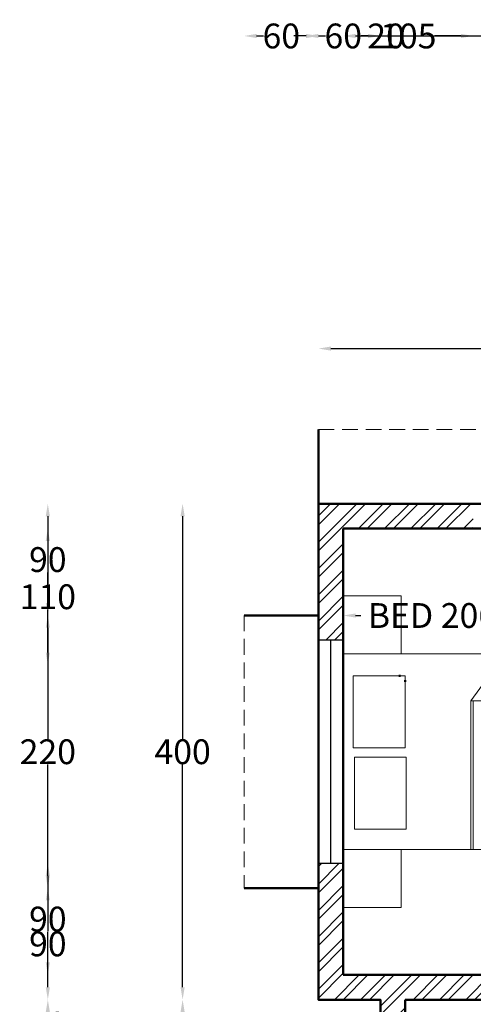
# Model space of a CAD drawing. Units: centimetres. Extents: x 10444 to 13814, y 8288 to 11191.
# Tile 4 of 9: x 10444 to 10810, y 10397 to 11191. Entities that reach past the tile are written whole.
import ezdxf

# ---------------------------------------------------------------- set-up
doc = ezdxf.new("R2010")
doc.units = ezdxf.units.CM
doc.header["$MEASUREMENT"] = 0
doc.linetypes.add('DASHED', pattern=[19.05, 12.7, -6.35])
for name, color, linetype, lineweight in [('A-ANNO-DIMS', 2, 'Continuous', 18), ('A-FURN', 8, 'Continuous', 18), ('A-GLAZ', 4, 'Continuous', 25), ('A-ROOF-OVHD', 6, 'DASHED', 18), ('A-WALL', 7, 'Continuous', 50), ('A-WALL-PATT', 8, 'Continuous', 13)]:
    doc.layers.add(name, color=color, linetype=linetype, lineweight=lineweight)
doc.styles.get("Standard").update_dxf_attribs({"font": 'arial.ttf'})
doc.dimstyles.get("Standard").update_dxf_attribs({"dimtxt": 20, "dimasz": 10, "dimexe": 0.18, "dimexo": 0.0625, "dimgap": 0.09, "dimtad": 0, "dimtih": 1, "dimtoh": 1, "dimdec": 0, "dimzin": 0, "dimdsep": 46, "dimtxsty": 'Standard', "dimcen": 0.09, "dimse1": 1, "dimse2": 1, "dimadec": 0, "dimazin": 0, "dimtfac": 1, "dimtdec": 0, "dimtofl": 0, "dimtmove": 0, "dimatfit": 3, "dimfxl": 1, "dimtolj": 1, "dimtzin": 0, "dimarcsym": 0})

# ---------------------------------------------------------------- blocks, each defined once
blk = doc.blocks.new('BED')
for p, q in [((1734.14, 2886.74), (1849.51, 2886.74)), ((1734.14, 2884.74), (1849.51, 2884.74)), ((1849.51, 2886.74), (1886.14, 2860.24)), ((1886.14, 2860.24), (1849.51, 2886.74)), ((1849.51, 2886.74), (1849.51, 2860.24)), ((1849.51, 2860.24), (1886.14, 2860.24))]:
    blk.add_line(p, q)
for points in [[(1734.14, 2787.74), (1886.14, 2787.74), (1886.14, 2985.74), (1734.14, 2985.74)], [(1749.96, 2936.84), (1805.89, 2936.84), (1805.89, 2977.01), (1749.96, 2977.01)], [(1813.22, 2937.77), (1869.15, 2937.77), (1869.15, 2977.94), (1813.22, 2977.94)]]:
    blk.add_lwpolyline(points, close=True)
blk = doc.blocks.new('*D10')
at = {"layer": 'A-ANNO-DIMS', "color": 0, "lineweight": -2, "transparency": 16777216}
for p, q in [((10694.79, 10925.83), (11210.81, 10925.83)), ((11784.79, 10925.83), (11268.77, 10925.83))]:
    blk.add_line(p, q, dxfattribs=at)
at = {"layer": 'A-ANNO-DIMS', "color": 0, "transparency": 16777216}
for points in [[(10694.79, 10927.49), (10694.79, 10924.16), (10684.79, 10925.83)], [(11784.79, 10927.49), (11784.79, 10924.16), (11794.79, 10925.83)]]:
    blk.add_solid(points, dxfattribs=at)
at = {"layer": 'Defpoints', "color": 0, "transparency": 16777216}
for p in [(11794.79, 10925.83), (10684.79, 10800.63), (11794.79, 10800.63)]:
    blk.add_point(p, dxfattribs=at)
at = {"layer": 'A-ANNO-DIMS', "color": 0, "transparency": 16777216, "insert": (11239.79, 10925.83), "char_height": 20, "attachment_point": 5}
blk.add_mtext('\\A1;1110', dxfattribs=at)
blk = doc.blocks.new('*D11')
at = {"layer": 'A-ANNO-DIMS', "color": 0, "lineweight": -2, "transparency": 16777216}
for p, q in [((10575.11, 10790.63), (10575.11, 10610.94)), ((10575.11, 10410.63), (10575.11, 10590.33))]:
    blk.add_line(p, q, dxfattribs=at)
at = {"layer": 'A-ANNO-DIMS', "color": 0, "transparency": 16777216}
for points in [[(10573.44, 10790.63), (10576.77, 10790.63), (10575.11, 10800.63)], [(10573.44, 10410.63), (10576.77, 10410.63), (10575.11, 10400.63)]]:
    blk.add_solid(points, dxfattribs=at)
at = {"layer": 'Defpoints', "color": 0, "transparency": 16777216}
for p in [(10684.79, 10800.63), (10575.11, 10400.63), (10684.79, 10400.63)]:
    blk.add_point(p, dxfattribs=at)
at = {"layer": 'A-ANNO-DIMS', "color": 0, "transparency": 16777216, "insert": (10575.11, 10600.63), "char_height": 20, "attachment_point": 5}
blk.add_mtext('\\A1;400', dxfattribs=at)
blk = doc.blocks.new('*D12')
at = {"layer": 'A-ANNO-DIMS', "color": 0, "lineweight": -2, "transparency": 16777216}
for p, q in [((10575.11, 10390.63), (10575.11, 10170.94)), ((10575.11, 9930.63), (10575.11, 10150.33))]:
    blk.add_line(p, q, dxfattribs=at)
at = {"layer": 'A-ANNO-DIMS', "color": 0, "transparency": 16777216}
for points in [[(10573.44, 10390.63), (10576.77, 10390.63), (10575.11, 10400.63)], [(10573.44, 9930.63), (10576.77, 9930.63), (10575.11, 9920.63)]]:
    blk.add_solid(points, dxfattribs=at)
at = {"layer": 'Defpoints', "color": 0, "transparency": 16777216}
for p in [(10734.79, 10400.63), (10575.11, 9920.63), (10734.79, 9920.63)]:
    blk.add_point(p, dxfattribs=at)
at = {"layer": 'A-ANNO-DIMS', "color": 0, "transparency": 16777216, "insert": (10575.11, 10160.63), "char_height": 20, "attachment_point": 5}
blk.add_mtext('\\A1;480', dxfattribs=at)
blk = doc.blocks.new('*D13')
at = {"layer": 'A-ANNO-DIMS', "color": 0, "lineweight": -2, "transparency": 16777216}
for p, q in [((10694.79, 9801.88), (10695.41, 9801.88)), ((10724.79, 9801.88), (10724.17, 9801.88))]:
    blk.add_line(p, q, dxfattribs=at)
at = {"layer": 'A-ANNO-DIMS', "color": 0, "transparency": 16777216}
for points in [[(10694.79, 9803.55), (10694.79, 9800.21), (10684.79, 9801.88)], [(10724.79, 9803.55), (10724.79, 9800.21), (10734.79, 9801.88)]]:
    blk.add_solid(points, dxfattribs=at)
at = {"layer": 'Defpoints', "color": 0, "transparency": 16777216}
for p in [(10684.79, 10400.63), (10734.79, 10400.63), (10684.79, 9801.88)]:
    blk.add_point(p, dxfattribs=at)
at = {"layer": 'A-ANNO-DIMS', "color": 0, "transparency": 16777216, "insert": (10709.79, 9801.88), "char_height": 20, "attachment_point": 5}
blk.add_mtext('\\A1;50', dxfattribs=at)
blk = doc.blocks.new('WIN-1800')
blk.add_line((0, 10), (180, 10))
blk.add_lwpolyline([(0, 0), (180, 0), (180, 20), (0, 20)], close=True)
blk = doc.blocks.new('*D41')
at = {"layer": 'A-ANNO-DIMS', "color": 0, "lineweight": -2, "transparency": 16777216}
for p, q in [((10714.79, 10710.51), (10719, 10710.51)), ((10900.6, 10710.51), (10896.39, 10710.51))]:
    blk.add_line(p, q, dxfattribs=at)
at = {"layer": 'A-ANNO-DIMS', "color": 0, "transparency": 16777216}
for points in [[(10714.79, 10712.17), (10714.79, 10708.84), (10704.79, 10710.51)], [(10900.6, 10712.17), (10900.6, 10708.84), (10910.6, 10710.51)]]:
    blk.add_solid(points, dxfattribs=at)
at = {"layer": 'Defpoints', "color": 0, "transparency": 16777216}
for p in [(10704.79, 10710.51), (10704.79, 10679.63), (10910.6, 10679.63)]:
    blk.add_point(p, dxfattribs=at)
at = {"layer": 'A-ANNO-DIMS', "color": 0, "transparency": 16777216, "insert": (10807.7, 10710.51), "char_height": 20, "attachment_point": 5}
blk.add_mtext('\\A1;BED 206 TYP.', dxfattribs=at)
blk = doc.blocks.new('*D51')
at = {"layer": 'A-ANNO-DIMS', "color": 0, "lineweight": -2, "transparency": 16777216}
for p, q in [((10674.79, 11178), (10664.79, 11178)), ((10714.79, 11178), (10724.79, 11178))]:
    blk.add_line(p, q, dxfattribs=at)
at = {"layer": 'A-ANNO-DIMS', "color": 0, "transparency": 16777216}
for points in [[(10674.79, 11179.67), (10674.79, 11176.33), (10684.79, 11178)], [(10714.79, 11179.67), (10714.79, 11176.33), (10704.79, 11178)]]:
    blk.add_solid(points, dxfattribs=at)
at = {"layer": 'Defpoints', "color": 0, "transparency": 16777216}
for p in [(10704.79, 11178), (10684.79, 10800.63), (10704.79, 10780.63)]:
    blk.add_point(p, dxfattribs=at)
at = {"layer": 'A-ANNO-DIMS', "color": 0, "transparency": 16777216, "insert": (10739.34, 11178), "char_height": 20, "attachment_point": 5}
blk.add_mtext('\\A1;20', dxfattribs=at)
blk = doc.blocks.new('*D52')
at = {"layer": 'A-ANNO-DIMS', "color": 0, "lineweight": -2, "transparency": 16777216}
for p, q in [((10714.79, 11178), (10735.97, 11178)), ((10799.79, 11178), (10778.61, 11178))]:
    blk.add_line(p, q, dxfattribs=at)
at = {"layer": 'A-ANNO-DIMS', "color": 0, "transparency": 16777216}
for points in [[(10714.79, 11179.67), (10714.79, 11176.33), (10704.79, 11178)], [(10799.79, 11179.67), (10799.79, 11176.33), (10809.79, 11178)]]:
    blk.add_solid(points, dxfattribs=at)
at = {"layer": 'Defpoints', "color": 0, "transparency": 16777216}
for p in [(10809.79, 11178), (10809.79, 10800.63), (10704.79, 10780.63)]:
    blk.add_point(p, dxfattribs=at)
at = {"layer": 'A-ANNO-DIMS', "color": 0, "transparency": 16777216, "insert": (10757.29, 11178), "char_height": 20, "attachment_point": 5}
blk.add_mtext('\\A1;105', dxfattribs=at)
blk = doc.blocks.new('*D60')
at = {"layer": 'A-ANNO-DIMS', "color": 0, "lineweight": -2, "transparency": 16777216}
for p, q in [((10466.29, 10790.63), (10466.29, 10765.94)), ((10466.29, 10720.63), (10466.29, 10745.33))]:
    blk.add_line(p, q, dxfattribs=at)
at = {"layer": 'A-ANNO-DIMS', "color": 0, "transparency": 16777216}
for points in [[(10464.62, 10790.63), (10467.95, 10790.63), (10466.29, 10800.63)], [(10464.62, 10720.63), (10467.95, 10720.63), (10466.29, 10710.63)]]:
    blk.add_solid(points, dxfattribs=at)
at = {"layer": 'Defpoints', "color": 0, "transparency": 16777216}
for p in [(10684.79, 10800.63), (10466.29, 10710.63), (10624.79, 10710.63)]:
    blk.add_point(p, dxfattribs=at)
at = {"layer": 'A-ANNO-DIMS', "color": 0, "transparency": 16777216, "insert": (10466.29, 10755.63), "char_height": 20, "attachment_point": 5}
blk.add_mtext('\\A1;90', dxfattribs=at)
blk = doc.blocks.new('*D61')
at = {"layer": 'A-ANNO-DIMS', "color": 0, "lineweight": -2, "transparency": 16777216}
for p, q in [((10466.29, 10700.63), (10466.29, 10610.94)), ((10466.29, 10500.63), (10466.29, 10590.33))]:
    blk.add_line(p, q, dxfattribs=at)
at = {"layer": 'A-ANNO-DIMS', "color": 0, "transparency": 16777216}
for points in [[(10464.62, 10700.63), (10467.95, 10700.63), (10466.29, 10710.63)], [(10464.62, 10500.63), (10467.95, 10500.63), (10466.29, 10490.63)]]:
    blk.add_solid(points, dxfattribs=at)
at = {"layer": 'Defpoints', "color": 0, "transparency": 16777216}
for p in [(10624.79, 10710.63), (10466.29, 10490.63), (10624.79, 10490.63)]:
    blk.add_point(p, dxfattribs=at)
at = {"layer": 'A-ANNO-DIMS', "color": 0, "transparency": 16777216, "insert": (10466.29, 10600.63), "char_height": 20, "attachment_point": 5}
blk.add_mtext('\\A1;220', dxfattribs=at)
blk = doc.blocks.new('*D62')
at = {"layer": 'A-ANNO-DIMS', "color": 0, "lineweight": -2, "transparency": 16777216}
for p, q in [((10466.29, 10480.63), (10466.29, 10455.94)), ((10466.29, 10410.63), (10466.29, 10435.33))]:
    blk.add_line(p, q, dxfattribs=at)
at = {"layer": 'A-ANNO-DIMS', "color": 0, "transparency": 16777216}
for points in [[(10464.62, 10480.63), (10467.95, 10480.63), (10466.29, 10490.63)], [(10464.62, 10410.63), (10467.95, 10410.63), (10466.29, 10400.63)]]:
    blk.add_solid(points, dxfattribs=at)
at = {"layer": 'Defpoints', "color": 0, "transparency": 16777216}
for p in [(10624.79, 10490.63), (10466.29, 10400.63), (10684.79, 10400.63)]:
    blk.add_point(p, dxfattribs=at)
at = {"layer": 'A-ANNO-DIMS', "color": 0, "transparency": 16777216, "insert": (10466.29, 10445.63), "char_height": 20, "attachment_point": 5}
blk.add_mtext('\\A1;90', dxfattribs=at)
blk = doc.blocks.new('*D63')
at = {"layer": 'A-ANNO-DIMS', "color": 0, "lineweight": -2, "transparency": 16777216}
for p, q in [((10466.29, 10410.63), (10466.29, 10420.63)), ((10466.29, 10350.63), (10466.29, 10340.63))]:
    blk.add_line(p, q, dxfattribs=at)
at = {"layer": 'A-ANNO-DIMS', "color": 0, "transparency": 16777216}
for points in [[(10464.62, 10410.63), (10467.95, 10410.63), (10466.29, 10400.63)], [(10464.62, 10350.63), (10467.95, 10350.63), (10466.29, 10360.63)]]:
    blk.add_solid(points, dxfattribs=at)
at = {"layer": 'Defpoints', "color": 0, "transparency": 16777216}
for p in [(10684.79, 10400.63), (10466.29, 10360.63), (10674.79, 10360.63)]:
    blk.add_point(p, dxfattribs=at)
at = {"layer": 'A-ANNO-DIMS', "color": 0, "transparency": 16777216, "insert": (10466.29, 10380.63), "char_height": 20, "attachment_point": 5}
blk.add_mtext('\\A1;40', dxfattribs=at)
blk = doc.blocks.new('*D68')
at = {"layer": 'A-ANNO-DIMS', "color": 0, "lineweight": -2, "transparency": 16777216}
for p, q in [((10714.79, 11178), (10877.64, 11178)), ((11084.79, 11178), (10921.93, 11178))]:
    blk.add_line(p, q, dxfattribs=at)
at = {"layer": 'A-ANNO-DIMS', "color": 0, "transparency": 16777216}
for points in [[(10714.79, 11179.67), (10714.79, 11176.33), (10704.79, 11178)], [(11084.79, 11179.67), (11084.79, 11176.33), (11094.79, 11178)]]:
    blk.add_solid(points, dxfattribs=at)
at = {"layer": 'Defpoints', "color": 0, "transparency": 16777216}
for p in [(11094.79, 11178), (10704.79, 10780.63), (11094.79, 10700.63)]:
    blk.add_point(p, dxfattribs=at)
at = {"layer": 'A-ANNO-DIMS', "color": 0, "transparency": 16777216, "insert": (10899.79, 11178), "char_height": 20, "attachment_point": 5}
blk.add_mtext('\\A1;390', dxfattribs=at)
blk = doc.blocks.new('*D71')
at = {"layer": 'A-ANNO-DIMS', "color": 0, "lineweight": -2, "transparency": 16777216}
for p, q in [((10466.29, 10770.63), (10466.29, 10735.94)), ((10466.29, 10680.63), (10466.29, 10715.33))]:
    blk.add_line(p, q, dxfattribs=at)
at = {"layer": 'A-ANNO-DIMS', "color": 0, "transparency": 16777216}
for points in [[(10464.62, 10770.63), (10467.95, 10770.63), (10466.29, 10780.63)], [(10464.62, 10680.63), (10467.95, 10680.63), (10466.29, 10670.63)]]:
    blk.add_solid(points, dxfattribs=at)
at = {"layer": 'Defpoints', "color": 0, "transparency": 16777216}
for p in [(11594.79, 10780.63), (10466.29, 10670.63), (11674.79, 10670.63)]:
    blk.add_point(p, dxfattribs=at)
at = {"layer": 'A-ANNO-DIMS', "color": 0, "transparency": 16777216, "insert": (10466.29, 10725.63), "char_height": 20, "attachment_point": 5}
blk.add_mtext('\\A1;110', dxfattribs=at)
blk = doc.blocks.new('*D75')
at = {"layer": 'A-ANNO-DIMS', "color": 0, "lineweight": -2, "transparency": 16777216}
for p, q in [((10466.29, 10500.63), (10466.29, 10475.94)), ((10466.29, 10430.63), (10466.29, 10455.33))]:
    blk.add_line(p, q, dxfattribs=at)
at = {"layer": 'A-ANNO-DIMS', "color": 0, "transparency": 16777216}
for points in [[(10464.62, 10500.63), (10467.95, 10500.63), (10466.29, 10510.63)], [(10464.62, 10430.63), (10467.95, 10430.63), (10466.29, 10420.63)]]:
    blk.add_solid(points, dxfattribs=at)
at = {"layer": 'Defpoints', "color": 0, "transparency": 16777216}
for p in [(10466.29, 10510.63), (11784.79, 10510.63), (11794.79, 10420.63)]:
    blk.add_point(p, dxfattribs=at)
at = {"layer": 'A-ANNO-DIMS', "color": 0, "transparency": 16777216, "insert": (10466.29, 10465.63), "char_height": 20, "attachment_point": 5}
blk.add_mtext('\\A1;90', dxfattribs=at)
blk = doc.blocks.new('*D76')
at = {"layer": 'A-ANNO-DIMS', "color": 0, "lineweight": -2, "transparency": 16777216}
for p, q in [((10466.29, 10390.63), (10466.29, 10360.94)), ((10466.29, 10310.63), (10466.29, 10340.33))]:
    blk.add_line(p, q, dxfattribs=at)
at = {"layer": 'A-ANNO-DIMS', "color": 0, "transparency": 16777216}
for points in [[(10464.62, 10390.63), (10467.95, 10390.63), (10466.29, 10400.63)], [(10464.62, 10310.63), (10467.95, 10310.63), (10466.29, 10300.63)]]:
    blk.add_solid(points, dxfattribs=at)
at = {"layer": 'Defpoints', "color": 0, "transparency": 16777216}
for p in [(10466.29, 10400.63), (11114.79, 10400.63), (11054.79, 10300.63)]:
    blk.add_point(p, dxfattribs=at)
at = {"layer": 'A-ANNO-DIMS', "color": 0, "transparency": 16777216, "insert": (10466.29, 10350.63), "char_height": 20, "attachment_point": 5}
blk.add_mtext('\\A1;100', dxfattribs=at)
blk = doc.blocks.new('*D77')
at = {"layer": 'A-ANNO-DIMS', "color": 0, "lineweight": -2, "transparency": 16777216}
for p, q in [((10634.79, 11178), (10640.35, 11178)), ((10674.79, 11178), (10669.22, 11178))]:
    blk.add_line(p, q, dxfattribs=at)
at = {"layer": 'A-ANNO-DIMS', "color": 0, "transparency": 16777216}
for points in [[(10634.79, 11179.67), (10634.79, 11176.33), (10624.79, 11178)], [(10674.79, 11179.67), (10674.79, 11176.33), (10684.79, 11178)]]:
    blk.add_solid(points, dxfattribs=at)
at = {"layer": 'Defpoints', "color": 0, "transparency": 16777216}
for p in [(10684.79, 11178), (10624.79, 10710.63), (10684.79, 10710.63)]:
    blk.add_point(p, dxfattribs=at)
at = {"layer": 'A-ANNO-DIMS', "color": 0, "transparency": 16777216, "insert": (10654.79, 11178), "char_height": 20, "attachment_point": 5}
blk.add_mtext('\\A1;60', dxfattribs=at)
blk = doc.blocks.new('*D78')
at = {"layer": 'A-ANNO-DIMS', "color": 0, "lineweight": -2, "transparency": 16777216}
for p, q in [((10684.79, 11178), (10690.35, 11178)), ((10724.79, 11178), (10719.22, 11178))]:
    blk.add_line(p, q, dxfattribs=at)
at = {"layer": 'A-ANNO-DIMS', "color": 0, "transparency": 16777216}
for points in [[(10684.79, 11179.67), (10684.79, 11176.33), (10674.79, 11178)], [(10724.79, 11179.67), (10724.79, 11176.33), (10734.79, 11178)]]:
    blk.add_solid(points, dxfattribs=at)
at = {"layer": 'Defpoints', "color": 0, "transparency": 16777216}
for p in [(10734.79, 11178), (10674.79, 10360.63), (10734.79, 10360.63)]:
    blk.add_point(p, dxfattribs=at)
at = {"layer": 'A-ANNO-DIMS', "color": 0, "transparency": 16777216, "insert": (10704.79, 11178), "char_height": 20, "attachment_point": 5}
blk.add_mtext('\\A1;60', dxfattribs=at)

msp = doc.modelspace()

# ---------------------------------------------------------------- hatches: boundary and pattern name
at = {"layer": 'A-WALL-PATT'}
h = msp.add_hatch(dxfattribs=at)
h.set_pattern_fill('ANSI32', color=256, scale=40)
h.paths.add_polyline_path([(10809.7881, 10800.6336), (10684.7881, 10800.6336), (10684.7881, 10690.6336), (10704.7881, 10690.6336), (10704.7881, 10726.41), (10704.7881, 10780.6336), (10809.7881, 10780.6336)])
h.paths.add_polyline_path([(11154.7881, 10800.6336), (10989.7881, 10800.6336), (10989.7881, 10780.6336), (11114.7881, 10780.6336), (11154.7881, 10780.6336)])
h.paths.add_polyline_path([(11354.7881, 10800.6336), (11214.7881, 10800.6336), (11214.7881, 10780.6336), (11254.7881, 10780.6336), (11254.7881, 10582.9925, -0.00499308), (11254.7881, 10581.0383), (11254.7881, 10571.0719, -0.26947312), (11256.5873, 10571.9821), (11256.5873, 10568.3227), (11256.5873, 10564.4272, -0.26947312), (11254.7881, 10565.3375), (11254.7881, 10530.6336), (11196.6819, 10530.6336), (11196.6819, 10510.6336), (11254.7881, 10510.6336), (11254.7881, 10400.6336), (11274.7881, 10400.6336), (11274.7881, 10420.6336), (11274.7881, 10780.6336), (11354.7881, 10780.6336)])
h.paths.add_polyline_path([(10704.7881, 10510.6336), (10684.7881, 10510.6336), (10684.7881, 10400.6336), (10734.7881, 10400.6336), (10734.7881, 10340.6336), (10754.7881, 10340.6336), (10754.7881, 10400.6336), (11114.7881, 10400.6336), (11114.7881, 10420.6336), (10704.7881, 10420.6336)])
h.paths.add_polyline_path([(11794.7881, 10420.6336), (11364.7881, 10420.6336), (11364.7881, 10400.6336), (11644.7881, 10400.6336), (11644.7881, 10260.6336), (11664.7881, 10260.6336), (11664.7881, 10400.6336), (11794.7881, 10400.6336)])
h.paths.add_polyline_path([(11594.7881, 10670.6336), (11594.7881, 10708.9482, -0.26828041), (11592.9938, 10708.0455), (11592.9938, 10711.9409), (11592.9938, 10715.6003, -0.26828041), (11594.7881, 10714.6976), (11594.7881, 10780.6336), (11654.7881, 10780.6336), (11654.7881, 10800.6336), (11494.7881, 10800.6336), (11494.7881, 10780.6336), (11574.7881, 10780.6336), (11574.7881, 10510.6336), (11594.7881, 10510.6336)])
h.paths.add_polyline_path([(11794.7881, 10800.6336), (11714.7881, 10800.6336), (11714.7881, 10780.6336), (11774.7881, 10780.6336), (11774.7881, 10750.6336), (11794.7881, 10750.6336)])
h.paths.add_polyline_path([(11794.7881, 10670.6336), (11674.7881, 10670.6336), (11674.7881, 10650.6336), (11794.7881, 10650.6336)])
h.paths.add_polyline_path([(11664.7881, 10080.6336), (11644.7881, 10080.6336), (11644.7881, 9940.6336), (11549.7881, 9940.6336), (11549.7881, 9920.6336), (11664.7881, 9920.6336)])
h.paths.add_polyline_path([(11369.7881, 9940.6336), (11274.7881, 9940.6336), (11274.7881, 10300.6336), (11254.7881, 10300.6336), (11254.7881, 9940.6336), (11234.7881, 9940.6336), (11234.7881, 9920.6336), (11369.7881, 9920.6336)])
h.paths.add_polyline_path([(11094.7881, 9940.6336), (11074.7881, 9940.6336), (11074.7881, 10300.6336), (11054.7881, 10300.6336), (11054.7881, 10080.6336), (11054.7881, 9920.6336), (11094.7881, 9920.6336)])
h.paths.add_polyline_path([(11134.7881, 9940.6336), (11114.7881, 9940.6336), (11114.7881, 9920.6336), (11134.7881, 9920.6336)])
h.paths.add_polyline_path([(11174.7881, 9940.6336), (11154.7881, 9940.6336), (11154.7881, 9920.6336), (11174.7881, 9920.6336)])
h.paths.add_polyline_path([(11214.7881, 9940.6336), (11196.6819, 9940.6336), (11196.6819, 9920.6336), (11214.7881, 9920.6336)])
h.paths.add_polyline_path([(10954.7881, 10100.6336), (10874.7881, 10100.6336), (10874.7881, 10080.6336), (10954.7881, 10080.6336)])
h.paths.add_polyline_path([(10814.7881, 10100.6336), (10754.7881, 10100.6336), (10754.7881, 10160.6336), (10734.7881, 10160.6336), (10734.7881, 10080.6336), (10814.7881, 10080.6336)])
h.paths.add_polyline_path([(11255.1494, 10331.8339), (11286.882, 10331.8339), (11286.882, 10373.0481), (11255.1494, 10373.0481)], flags=9)
h.paths.add_polyline_path([(11607.8445, 10630.7128), (11653.5607, 10630.7128), (11653.5607, 10671.927), (11607.8445, 10671.927)], flags=25)
h.paths.add_polyline_path([(11746.8445, 10447.0791), (11792.5607, 10447.0791), (11792.5607, 10488.2933), (11746.8445, 10488.2933)], flags=9)
h.paths.add_polyline_path([(11296.8445, 10388.5791), (11342.5607, 10388.5791), (11342.5607, 10429.7933), (11296.8445, 10429.7933)], flags=9)
h.paths.add_polyline_path([(11376.6416, 10156.0222), (11521.6757, 10156.0222), (11521.6757, 10230.6515), (11376.6416, 10230.6515)], flags=9)
h.paths.add_polyline_path([(11437.3982, 10313.4478), (11545.1881, 10313.4478), (11545.1881, 10354.662), (11437.3982, 10354.662)], flags=25)
h.paths.add_polyline_path([(11655.4027, 10682.0329), (11777.2718, 10682.0329), (11777.2718, 10756.6623), (11655.4027, 10756.6623)], flags=9)
h.paths.add_polyline_path([(11636.2626, 10500.0811), (11758.1316, 10500.0811), (11758.1316, 10574.7105), (11636.2626, 10574.7105)], flags=9)
h.paths.add_polyline_path([(11336.6251, 10562.3234), (11469.2581, 10562.3234), (11469.2581, 10636.9528), (11336.6251, 10636.9528)], flags=9)

# ---------------------------------------------------------------- linework, layer by layer
at = {"layer": 'A-FURN'}
for points in [[(10704.7881, 10726.41), (10704.7881, 10679.6336), (10751.5644, 10679.6336), (10751.5644, 10726.41)], [(10704.7881, 10521.6336), (10704.7881, 10474.8573), (10751.5644, 10474.8573), (10751.5644, 10521.6336)]]:
    msp.add_lwpolyline(points, close=True, dxfattribs=at)
at = {"layer": 'A-ROOF-OVHD'}
for p, q in [((10684.7881, 10860.6336), (11854.7881, 10860.6336)), ((10624.7881, 10710.6336), (10624.7881, 10490.6336))]:
    msp.add_line(p, q, dxfattribs=at)
at = {"layer": 'A-WALL'}
for p, q in [((10684.7881, 10860.6336), (10684.7881, 10400.6336)), ((10684.7881, 10800.6336), (11794.7881, 10800.6336)), ((10704.7881, 10780.6336), (10704.7881, 10420.6336)), ((10704.7881, 10780.6336), (11114.7881, 10780.6336)), ((10684.7881, 10710.6336), (10624.7881, 10710.6336)), ((10684.7881, 10690.6336), (10684.7881, 10710.6336)), ((10751.0978, 10661.9703), (10749.6557, 10661.9703)), ((10754.6557, 10658.4124), (10754.6557, 10656.9703)), ((10684.7881, 10510.6336), (10684.7881, 10490.6336)), ((10684.7881, 10490.6336), (10624.7881, 10490.6336)), ((10704.7881, 10420.6336), (11114.7881, 10420.6336)), ((10684.7881, 10400.6336), (10734.7881, 10400.6336)), ((10734.7881, 10400.6336), (10734.7881, 9940.6336)), ((10754.7881, 10400.6336), (11114.7881, 10400.6336)), ((10754.7881, 10400.6336), (10754.7881, 10100.6336))]:
    msp.add_line(p, q, dxfattribs=at)
msp.add_lwpolyline([(10734.7881, 9920.6336), (11664.7881, 9920.6336), (11664.7881, 10400.6336), (11794.7881, 10400.6336), (11794.7881, 10800.6336), (10684.7881, 10800.6336), (10684.7881, 10400.6336), (10734.7881, 10400.6336), (10734.7881, 9920.6336)], dxfattribs=at)

# ---------------------------------------------------------------- block references
at = {"layer": 'A-FURN', "xscale": 1.039473684210526, "yscale": 1.039473684210526, "zscale": 1.039473684210526, "rotation": 89.99999999999999}
msp.add_blockref('BED', (13808.3851, 8719.0411), dxfattribs=at)
at = {"layer": 'A-GLAZ', "rotation": 90.00000000000067}
msp.add_blockref('WIN-1800', (10704.7877, 10510.6335), dxfattribs=at)

# ---------------------------------------------------------------- dimensions: what is measured, and where the dimension line sits
at = {"layer": 'A-ANNO-DIMS'}
for base, p1, p2, picture, middle in [((10684.7881, 11178), (10624.7881, 10710.6336), (10684.7881, 10710.6336), '*D77', (10654.7881, 11178)), ((10704.7881, 11178), (10684.7881, 10800.6336), (10704.7881, 10780.6336), '*D51', (10739.3392, 11178)), ((10734.7881, 11178), (10674.7881, 10360.6336), (10734.7881, 10360.6336), '*D78', (10704.7881, 11178)), ((10809.7881, 11178), (10704.7881, 10780.6336), (10809.7881, 10800.6336), '*D52', (10757.2881, 11178)), ((11094.7881, 11178), (10704.7881, 10780.6336), (11094.7881, 10700.6336), '*D68', (10899.7881, 11178))]:
    dim = msp.add_linear_dim(base=base, p1=p1, p2=p2, dimstyle='Standard', override={"dimdec": 0, "dimlfac": 1, "dimrnd": 0, "dimzin": 0, "dimdsep": 46, "dimlunit": 2}, dxfattribs=at)
    dim.commit()
    dim.dimension.update_dxf_attribs({"geometry": picture, "text_midpoint": middle})
for p1, p2, distance, picture, middle in [((10684.7881, 10800.6336), (11794.7881, 10800.6336), 125.1941, '*D10', (11239.7881, 10925.8277)), ((10684.7881, 10800.6336), (10684.7881, 10400.6336), -109.6819, '*D11', (10575.1062, 10600.6336)), ((10734.7881, 10400.6336), (10734.7881, 9920.6336), -159.6819, '*D12', (10575.1062, 10160.6336)), ((10734.7881, 10400.6336), (10684.7881, 10400.6336), 598.7533, '*D13', (10709.7881, 9801.8804))]:
    dim = msp.add_aligned_dim(p1=p1, p2=p2, distance=distance, dimstyle='Standard', override={"dimclrd": 0, "dimclre": 0, "dimclrt": 0}, dxfattribs=at)
    dim.commit()
    dim.dimension.update_dxf_attribs({"geometry": picture, "text_midpoint": middle})
for base, p1, p2, picture, middle in [((10466.2881, 10710.6336), (10684.7881, 10800.6336), (10624.7881, 10710.6336), '*D60', (10466.2881, 10755.6336)), ((10466.2881, 10670.6336), (11594.7881, 10780.6336), (11674.7881, 10670.6336), '*D71', (10466.2881, 10725.6336)), ((10466.2881, 10490.6336), (10624.7881, 10710.6336), (10624.7881, 10490.6336), '*D61', (10466.2881, 10600.6336)), ((10466.2881, 10510.6336), (11794.7881, 10420.6336), (11784.7881, 10510.6336), '*D75', (10466.2881, 10465.6336)), ((10466.2881, 10400.6336), (10624.7881, 10490.6336), (10684.7881, 10400.6336), '*D62', (10466.2881, 10445.6336)), ((10466.2881, 10360.6336), (10684.7881, 10400.6336), (10674.7881, 10360.6336), '*D63', (10466.2881, 10380.6336)), ((10466.2881, 10400.6336), (11054.7881, 10300.6336), (11114.7881, 10400.6336), '*D76', (10466.2881, 10350.6336))]:
    dim = msp.add_linear_dim(base=base, p1=p1, p2=p2, angle=90, dimstyle='Standard', override={"dimdec": 0, "dimlfac": 1, "dimrnd": 0, "dimzin": 0, "dimdsep": 46, "dimlunit": 2}, dxfattribs=at)
    dim.commit()
    dim.dimension.update_dxf_attribs({"geometry": picture, "text_midpoint": middle})
dim = msp.add_linear_dim(base=(10704.7881, 10710.506), p1=(10910.6039, 10679.6336), p2=(10704.7881, 10679.6336), angle=180, text='BED <> TYP.', dimstyle='Standard', override={"dimdec": 0, "dimrnd": 0, "dimzin": 0, "dimlunit": 2}, dxfattribs=at)
dim.commit()
dim.dimension.update_dxf_attribs({"geometry": '*D41', "text_midpoint": (10807.696, 10710.506)})

doc.saveas('drawing.dxf')
